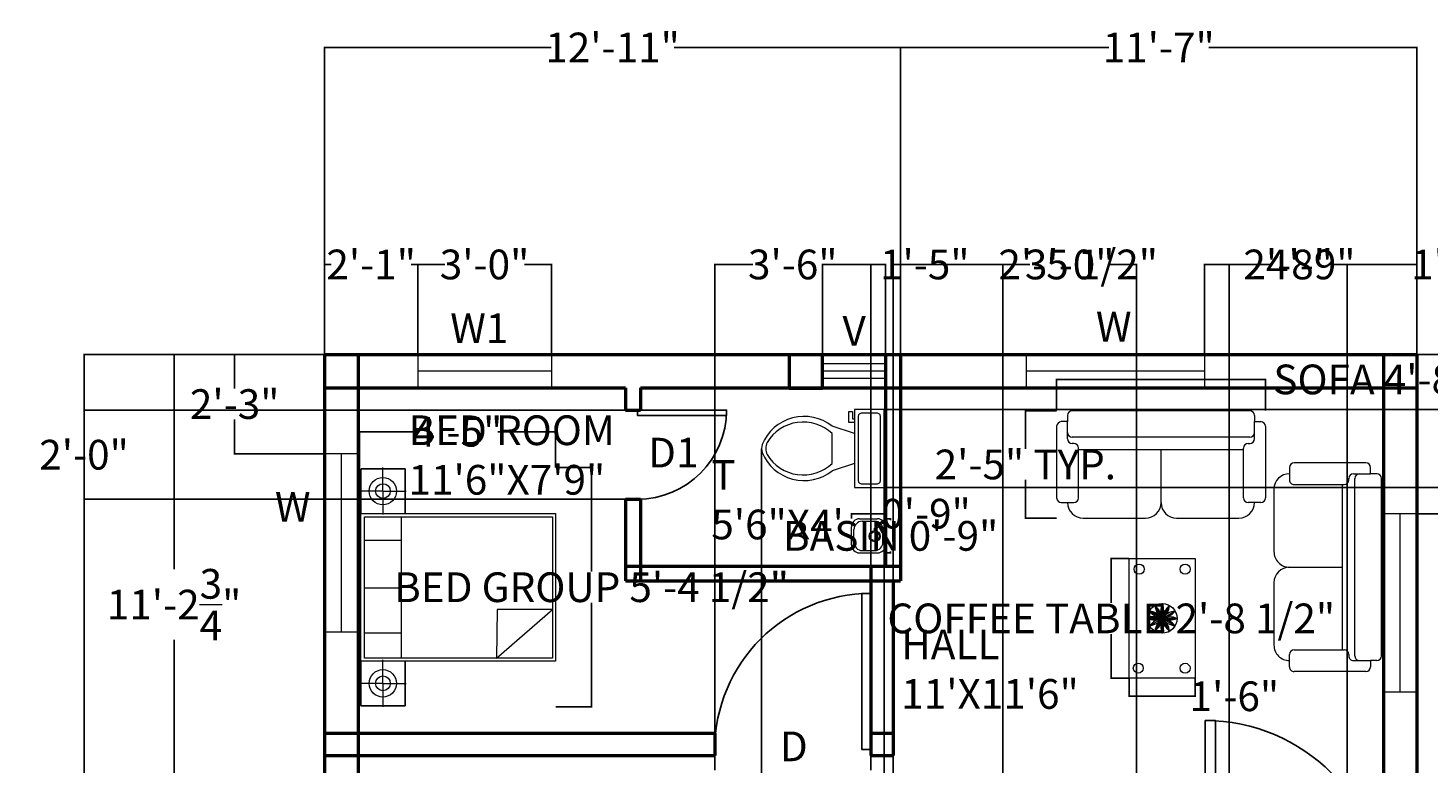
# Model space of a CAD drawing. Units: inches. Extents: x 1305 to 1889, y -508 to -5.
# Tile 7 of 8: x 1314 to 1691, y -220 to -22. Entities that reach past the tile are written whole.
import ezdxf

# ---------------------------------------------------------------- set-up
doc = ezdxf.new("R2010")
doc.units = ezdxf.units.IN
doc.header["$MEASUREMENT"] = 0
for name, color, linetype, lineweight in [('A-ANNO-DIMS', 2, 'Continuous', 18), ('A-ANNO-TEXT', 7, 'Continuous', 18), ('A-AREA-IDEN', 7, 'Continuous', 25), ('A-COLS', 7, 'Continuous', 50), ('A-DOOR', 3, 'Continuous', 25), ('A-FLOR-FIXT', 9, 'Continuous', 18), ('A-FURN', 8, 'Continuous', 18), ('A-GLAZ', 4, 'Continuous', 18), ('A-WALL', 7, 'Continuous', 50)]:
    doc.layers.add(name, color=color, linetype=linetype, lineweight=lineweight)
doc.styles.get("Standard").update_dxf_attribs({"font": 'arial.ttf', "height": 8})
doc.dimstyles.get("Standard").update_dxf_attribs({"dimtxt": 0.18, "dimasz": 0.18, "dimexe": 0.18, "dimexo": 0.0625, "dimgap": 0.09, "dimtad": 0, "dimtih": 1, "dimtoh": 1, "dimzin": 0, "dimdsep": 46, "dimlunit": 4, "dimtxsty": 'Standard', "dimcen": 0.09, "dimadec": 0, "dimazin": 0, "dimtfac": 1, "dimtofl": 0, "dimtmove": 0, "dimatfit": 3, "dimfxl": 1, "dimtolj": 1, "dimtzin": 0, "dimarcsym": 0})

# ---------------------------------------------------------------- blocks, each defined once
blk = doc.blocks.new('*U13')
for p, q in [((0, 0), (0, -100)), ((750, 0), (750, -100))]:
    blk.add_line(p, q)
blk.add_lwpolyline([(0, 0), (0, 750), (43.75, 750), (43.75, 0)], close=True)
blk.add_arc((0, 0), 750, 0, 90)
blk = doc.blocks.new('*U14')
for p, q in [((-750, 0), (-750, -100)), ((0, 0), (0, -100))]:
    blk.add_line(p, q)
blk.add_lwpolyline([(0, 0), (0, 750), (-43.75, 750), (-43.75, 0)], close=True)
blk.add_arc((0, 0), 750, 90, 180)
blk = doc.blocks.new('*U12')
for p, q in [((9.5, -6), (9.5, -2)), ((-10, -8.5), (-8, -8.5)), ((-10, -9.5), (-10, -8.5)), ((-7, -9.5), (-10, -9.5)), ((-8, -8.5), (-8, -8)), ((-7, -8), (-7, -9.5)), ((-4, -8), (-6, -14)), ((4, -8), (6, -14)), ((4, -14), (-4, -14))]:
    blk.add_line(p, q)
blk.add_lwpolyline([(10.5, -8), (10.5, 0), (-10.5, 0), (-10.5, -8)], close=True)
for points in [[(-9.5, -2), (-9.5, -6)], [(8.5, -1), (-8.5, -1)], [(-8.5, -7), (8.5, -7)]]:
    blk.add_lwpolyline(points)
for centre, radius, start, end in [((-8.62, -1.88), 0.884, 81.8699, 188.1301), ((8.62, -1.88), 0.884, 351.8699, 98.1301), ((-8.62, -6.12), 0.884, 171.8699, 278.1301), ((8.62, -6.12), 0.884, 261.8699, 8.1301), ((3.52, -21.58), 12.17, 141.4691, 247.9714), ((4.2, -21.82), 11.33, 136.3677, 238.9468), ((-3.52, -21.58), 12.17, 292.0284, 38.5307), ((-4.2, -21.82), 11.33, 301.053, 43.6321), ((0, -27.88), 4, 245.7318, 294.2682), ((0, -29), 4, 254.8605, 285.1395)]:
    blk.add_arc(centre, radius, start, end)
blk = doc.blocks.new('A$C027E3DAA')
for p, q in [((48, 356), (128, 276)), ((142, 290), (63, 369)), ((320, 420), (100, 420)), ((291, 388), (131, 388)), ((0, 100), (0, 320)), ((31, 132), (31, 288)), ((128, 276), (142, 290)), ((391, 132), (391, 288)), ((420, 100), (420, 320)), ((291, 32), (131, 32)), ((320, 0), (100, 0))]:
    blk.add_line(p, q)
for centre, radius in [((47, 373), 16.5), ((47, 373), 8.24), ((214, 287), 68.5), ((214, 287), 54.8)]:
    blk.add_circle(centre, radius)
for centre, start, end in [((100, 320), 90, 180), ((131, 288), 90, 180), ((291, 288), 0, 90), ((320, 320), 0, 90), ((100, 100), 180, 270), ((131, 132), 180, 270), ((291, 132), 270, 0), ((320, 100), 270, 0)]:
    blk.add_arc(centre, 100, start, end)
blk = doc.blocks.new('A$C214F6537')
for p, q in [((0.238, 1.755, -0.439), (0.238, 1.993, -0.439)), ((2.192, 1.755, -0.439), (2.192, 1.993, -0.439)), ((0.465, 1.98, -0.169), (0.011, 1.98, -0.169)), ((0.011, 1.98, -0.169), (0.011, 1.53, -0.169)), ((0.011, 1.98, -0.169), (2.419, 1.98, -0.169)), ((0.011, 1.53, -0.169), (0.011, 1.98, -0.169)), ((0.465, 0, -0.169), (0.465, 1.98, -0.169)), ((0.465, 1.98, -0.169), (1.965, 1.98, -0.169)), ((0.465, 1.53, -0.169), (0.465, 1.98, -0.169)), ((0.495, 1.941, -0.169), (1.929, 1.941, -0.169)), ((0.495, 1.57, -0.169), (0.495, 1.941, -0.169)), ((0.752, 1.941, -0.169), (0.752, 1.57, -0.169)), ((1.209, 1.941, -0.169), (1.209, 1.57, -0.169)), ((1.694, 1.941, -0.169), (1.694, 1.57, -0.169)), ((1.929, 1.941, -0.169), (1.929, 1.57, -0.169)), ((1.965, 1.98, -0.169), (1.965, 0, -0.169)), ((2.419, 1.98, -0.169), (1.965, 1.98, -0.169)), ((1.965, 1.98, -0.169), (1.965, 1.53, -0.169)), ((2.419, 1.53, -0.169), (2.419, 1.98, -0.169)), ((2.419, 1.98, -0.169), (2.419, 1.53, -0.169)), ((0.238, 1.755, -0.439), (0, 1.755, -0.439)), ((0.238, 1.755, -0.439), (0.238, 1.517, -0.439)), ((0.238, 1.755, -0.439), (0.476, 1.755, -0.439)), ((2.192, 1.755, -0.439), (1.954, 1.755, -0.439)), ((2.192, 1.755, -0.439), (2.43, 1.755, -0.439)), ((2.192, 1.755, -0.439), (2.192, 1.517, -0.439)), ((0.495, 0.032, -0.169), (0.495, 1.57, -0.169)), ((1.929, 1.57, -0.169), (0.495, 1.57, -0.169)), ((1.929, 1.57, -0.169), (1.929, 0.032, -0.169)), ((0.011, 1.53, -0.169), (0.465, 1.53, -0.169)), ((0.465, 1.53, -0.169), (0.011, 1.53, -0.169)), ((0.465, 0, -0.169), (0.465, 1.53, -0.169)), ((1.965, 1.53, -0.169), (2.419, 1.53, -0.169)), ((2.419, 1.53, -0.169), (1.965, 1.53, -0.169)), ((1.965, 1.53, -0.169), (1.965, 0, -0.169)), ((0.495, 0.6, -0.169), (0.987, 0.032, -0.169)), ((0.987, 0.595, -0.169), (0.495, 0.6, -0.169)), ((0.987, 0.032, -0.169), (0.987, 0.595, -0.169)), ((1.965, 0, -0.169), (0.465, 0, -0.169)), ((1.965, 0, -0.169), (0.465, 0, -0.169)), ((1.929, 0.032, -0.169), (0.495, 0.032, -0.169))]:
    blk.add_line(p, q)
for centre, radius in [((0.238, 1.755, -0.439), 0.139), ((2.192, 1.755, -0.439), 0.139), ((0.238, 1.755, -0.439), 0.075), ((2.192, 1.755, -0.439), 0.075)]:
    blk.add_circle(centre, radius)
blk = doc.blocks.new('A$C02A636C4')
for p, q in [((0.0679, 0.6401), (0.0679, 0.6013)), ((1.2026, 0.6692), (0.097, 0.6692)), ((1.2317, 0.6401), (1.2317, 0.6013)), ((0, 0.5722), (0, 0.1261)), ((0.0679, 0.6013), (0.0291, 0.6013)), ((0.0679, 0.5334), (0.0679, 0.6013)), ((0.0679, 0.4946), (0.0679, 0.5431)), ((1.2317, 0.6013), (1.2705, 0.6013)), ((1.2317, 0.5334), (1.2317, 0.6013)), ((1.2317, 0.4946), (1.2317, 0.5431)), ((1.2996, 0.5722), (1.2996, 0.1261)), ((1.2026, 0.5043), (0.097, 0.5043)), ((0.1067, 0.4655), (0.097, 0.4655)), ((0.1358, 0.1261), (0.1358, 0.4364)), ((1.1638, 0.1261), (1.1638, 0.4364)), ((1.1929, 0.4655), (1.2026, 0.4655)), ((1.1638, 0.4267), (0.1358, 0.4267)), ((0.6498, 0.097), (0.6498, 0.4267)), ((0.0291, 0.097), (0.1067, 0.097)), ((1.2705, 0.097), (1.1929, 0.097)), ((0.1649, 0), (0.5528, 0)), ((0.7468, 0), (1.1347, 0))]:
    blk.add_line(p, q)
for centre, radius, start, end in [((0.097, 0.6401), 0.0291, 90, 180), ((1.2026, 0.6401), 0.0291, 0, 90), ((0.0291, 0.5722), 0.0291, 90, 180), ((0.097, 0.5334), 0.0291, 180, 270), ((1.2026, 0.5334), 0.0291, 270, 0), ((1.2705, 0.5722), 0.0291, 0, 90), ((0.097, 0.4946), 0.0291, 180, 270), ((0.1067, 0.4364), 0.0291, 0, 90), ((1.1929, 0.4364), 0.0291, 90, 180), ((1.2026, 0.4946), 0.0291, 270, 0), ((0.0291, 0.1261), 0.0291, 180, 270), ((0.1649, 0.097), 0.097, 180, 270), ((0.1067, 0.1261), 0.0291, 270, 0), ((0.5528, 0.097), 0.097, 270, 0), ((0.7468, 0.097), 0.097, 180, 270), ((1.1347, 0.097), 0.097, 270, 0), ((1.1929, 0.1261), 0.0291, 180, 270), ((1.2705, 0.1261), 0.0291, 270, 0)]:
    blk.add_arc(centre, radius, start, end)
blk = doc.blocks.new('table')
blk.add_lwpolyline([(-20.55, 0), (36.33, 0), (36.33, -31.34), (-20.55, -31.34)], close=True)
for centre in [(-15.51, -4.83), (31.56, -4.83), (-15.51, -26.62), (31.48, -27.03)]:
    blk.add_circle(centre, 2.38)
blk = doc.blocks.new('*U18')
for p, q in [((3.98, 7.97), (3.98, 0)), ((0, 3.98), (7.97, 3.98))]:
    blk.add_line(p, q)
blk.add_circle((3.98, 3.98), 3.98)
for centre, start, end in [((8.79, 5.97), 157.5, 202.5), ((-0.82, 5.97), 337.5, 22.5), ((1.99, -0.82), 67.5, 112.5), ((1.99, 8.79), 247.5, 292.5), ((8.79, 1.99), 157.5, 202.5), ((5.97, -0.82), 67.5, 112.5), ((5.97, 8.79), 247.5, 292.5), ((-0.82, 1.99), 337.5, 22.5)]:
    blk.add_arc(centre, 5.2, start, end)
blk = doc.blocks.new('*U19')
at = {"layer": 'A-FURN', "color": 0, "linetype": 'ByBlock', "lineweight": -2, "transparency": 16777216}
for p, rotation in [((1620.98, -186.76), 60), ((1624.96, -182.78), 120), ((1618.06, -175.88), 240), ((1614.08, -179.87), 300), ((1623.5, -177.34), 180)]:
    blk.add_blockref('*U18', p, dxfattribs=dict(at, rotation=rotation))
blk.add_blockref('*U18', (1615.54, -185.31), dxfattribs=at)
blk = doc.blocks.new('*D20')
at = {"layer": 'A-ANNO-DIMS', "color": 0, "lineweight": -2, "transparency": 16777216}
for p, q in [((1394.01, -110.24), (1353.36, -110.24)), ((1353.54, -110.42), (1353.54, -168.1)), ((1353.54, -244.8), (1353.54, -187.12)), ((1394.01, -244.98), (1353.36, -244.98))]:
    blk.add_line(p, q, dxfattribs=at)
at = {"layer": 'A-ANNO-DIMS', "color": 0, "transparency": 16777216}
for points in [[(1353.51, -110.42), (1353.57, -110.42), (1353.54, -110.24)], [(1353.51, -244.8), (1353.57, -244.8), (1353.54, -244.98)]]:
    blk.add_solid(points, dxfattribs=at)
at = {"layer": 'Defpoints', "color": 0, "transparency": 16777216}
for p in [(1394.07, -110.24), (1353.54, -244.98), (1394.07, -244.98)]:
    blk.add_point(p, dxfattribs=at)
at = {"layer": 'A-ANNO-DIMS', "color": 0, "transparency": 16777216, "insert": (1353.54, -177.61), "char_height": 8, "attachment_point": 5}
blk.add_mtext('\\A1;11\'-2{\\H1x;\\S3/4;}"', dxfattribs=at)
blk = doc.blocks.new('*D25')
at = {"layer": 'A-ANNO-DIMS', "color": 0, "lineweight": -2, "transparency": 16777216}
for p, q in [((1394.07, -110.18), (1394.07, -27.4)), ((1394.25, -27.58), (1455.01, -27.58)), ((1548.89, -27.58), (1488.14, -27.58)), ((1549.07, -110.18), (1549.07, -27.4))]:
    blk.add_line(p, q, dxfattribs=at)
at = {"layer": 'A-ANNO-DIMS', "color": 0, "transparency": 16777216}
for points in [[(1394.25, -27.55), (1394.25, -27.61), (1394.07, -27.58)], [(1548.89, -27.55), (1548.89, -27.61), (1549.07, -27.58)]]:
    blk.add_solid(points, dxfattribs=at)
at = {"layer": 'Defpoints', "color": 0, "transparency": 16777216}
for p in [(1549.07, -27.58), (1394.07, -110.24), (1549.07, -110.24)]:
    blk.add_point(p, dxfattribs=at)
at = {"layer": 'A-ANNO-DIMS', "color": 0, "transparency": 16777216, "insert": (1471.57, -27.58), "char_height": 8, "attachment_point": 5}
blk.add_mtext('\\A1;12\'-11"', dxfattribs=at)
blk = doc.blocks.new('*D26')
at = {"layer": 'A-ANNO-DIMS', "color": 0, "lineweight": -2, "transparency": 16777216}
for p, q in [((1549.07, -110.18), (1549.07, -27.4)), ((1549.25, -27.58), (1605.12, -27.58)), ((1687.89, -27.58), (1632.03, -27.58)), ((1688.07, -110.18), (1688.07, -27.4))]:
    blk.add_line(p, q, dxfattribs=at)
at = {"layer": 'A-ANNO-DIMS', "color": 0, "transparency": 16777216}
for points in [[(1549.25, -27.55), (1549.25, -27.61), (1549.07, -27.58)], [(1687.89, -27.55), (1687.89, -27.61), (1688.07, -27.58)]]:
    blk.add_solid(points, dxfattribs=at)
at = {"layer": 'Defpoints', "color": 0, "transparency": 16777216}
for p in [(1688.07, -27.58), (1549.07, -110.24), (1688.07, -110.24)]:
    blk.add_point(p, dxfattribs=at)
at = {"layer": 'A-ANNO-DIMS', "color": 0, "transparency": 16777216, "insert": (1618.57, -27.58), "char_height": 8, "attachment_point": 5}
blk.add_mtext('\\A1;11\'-7"', dxfattribs=at)
blk = doc.blocks.new('WIN-48IN')
for p, q in [((0, 9), (0, 0)), ((48, 9), (48, 0)), ((48, 4.5), (0, 4.5))]:
    blk.add_line(p, q)
blk = doc.blocks.new('COL-9X9')
blk.add_lwpolyline([(0, 0), (9, 0), (9, 9), (0, 9)], close=True)
blk = doc.blocks.new('*D36')
at = {"layer": 'A-ANNO-DIMS', "color": 0, "lineweight": -2, "transparency": 16777216}
for p, q in [((1545.09, -154.5), (1546.59, -154.5)), ((1546.41, -154.68), (1546.41, -154.87)), ((1545.09, -163.69), (1546.59, -163.69)), ((1546.41, -163.51), (1546.41, -163.32))]:
    blk.add_line(p, q, dxfattribs=at)
at = {"layer": 'A-ANNO-DIMS', "color": 0, "transparency": 16777216}
for points in [[(1546.38, -154.68), (1546.44, -154.68), (1546.41, -154.5)], [(1546.38, -163.51), (1546.44, -163.51), (1546.41, -163.69)]]:
    blk.add_solid(points, dxfattribs=at)
at = {"layer": 'Defpoints', "color": 0, "transparency": 16777216}
for p in [(1545.03, -154.5), (1545.03, -163.69), (1546.41, -163.69)]:
    blk.add_point(p, dxfattribs=at)
at = {"layer": 'A-ANNO-DIMS', "color": 0, "transparency": 16777216, "insert": (1546.41, -159.1), "char_height": 8, "attachment_point": 5}
blk.add_mtext('\\A1;BASIN 0\'-9"', dxfattribs=at)
blk = doc.blocks.new('*D37')
at = {"layer": 'A-ANNO-DIMS', "color": 0, "lineweight": -2, "transparency": 16777216}
for p, q in [((1535.85, -154.44), (1535.85, -152.94)), ((1536.03, -153.12), (1544.85, -153.12)), ((1545.03, -154.44), (1545.03, -152.94)), ((1545.03, -153.12), (1545.21, -153.12))]:
    blk.add_line(p, q, dxfattribs=at)
at = {"layer": 'A-ANNO-DIMS', "color": 0, "transparency": 16777216}
for points in [[(1536.03, -153.09), (1536.03, -153.15), (1535.85, -153.12)], [(1544.85, -153.09), (1544.85, -153.15), (1545.03, -153.12)]]:
    blk.add_solid(points, dxfattribs=at)
at = {"layer": 'Defpoints', "color": 0, "transparency": 16777216}
for p in [(1545.03, -153.12), (1535.85, -154.5), (1545.03, -154.5)]:
    blk.add_point(p, dxfattribs=at)
at = {"layer": 'A-ANNO-DIMS', "color": 0, "transparency": 16777216, "insert": (1555.93, -153.12), "char_height": 8, "attachment_point": 5}
blk.add_mtext('\\A1;0\'-9"', dxfattribs=at)
blk = doc.blocks.new('*D38')
at = {"layer": 'A-ANNO-DIMS', "color": 0, "lineweight": -2, "transparency": 16777216}
for p, q in [((1591.1, -125.34), (1591.1, -116.79)), ((1647.29, -125.34), (1647.29, -116.79)), ((1591.28, -116.97), (1647.11, -116.97)), ((1647.29, -116.97), (1647.47, -116.97))]:
    blk.add_line(p, q, dxfattribs=at)
at = {"layer": 'A-ANNO-DIMS', "color": 0, "transparency": 16777216}
for points in [[(1591.28, -116.94), (1591.28, -117), (1591.1, -116.97)], [(1647.11, -116.94), (1647.11, -117), (1647.29, -116.97)]]:
    blk.add_solid(points, dxfattribs=at)
at = {"layer": 'Defpoints', "color": 0, "transparency": 16777216}
for p in [(1647.29, -116.97), (1591.1, -125.4), (1647.29, -125.4)]:
    blk.add_point(p, dxfattribs=at)
at = {"layer": 'A-ANNO-DIMS', "color": 0, "transparency": 16777216, "insert": (1688.69, -116.97), "char_height": 8, "attachment_point": 5}
blk.add_mtext('\\A1;SOFA 4\'-8" TYP.', dxfattribs=at)
blk = doc.blocks.new('*D39')
at = {"layer": 'A-ANNO-DIMS', "color": 0, "lineweight": -2, "transparency": 16777216}
for p, q in [((1591.04, -125.4), (1582.49, -125.4)), ((1582.67, -125.58), (1582.67, -135.7)), ((1582.67, -154.16), (1582.67, -144.04)), ((1591.04, -154.34), (1582.49, -154.34))]:
    blk.add_line(p, q, dxfattribs=at)
at = {"layer": 'A-ANNO-DIMS', "color": 0, "transparency": 16777216}
for points in [[(1582.64, -125.58), (1582.7, -125.58), (1582.67, -125.4)], [(1582.64, -154.16), (1582.7, -154.16), (1582.67, -154.34)]]:
    blk.add_solid(points, dxfattribs=at)
at = {"layer": 'Defpoints', "color": 0, "transparency": 16777216}
for p in [(1582.67, -125.4), (1591.1, -125.4), (1591.1, -154.34)]:
    blk.add_point(p, dxfattribs=at)
at = {"layer": 'A-ANNO-DIMS', "color": 0, "transparency": 16777216, "insert": (1582.67, -139.87), "char_height": 8, "attachment_point": 5}
blk.add_mtext('\\A1;2\'-5" TYP.', dxfattribs=at)
blk = doc.blocks.new('*D46')
at = {"layer": 'A-ANNO-DIMS', "color": 0, "lineweight": -2, "transparency": 16777216}
for p, q in [((1456.31, -140.72), (1466.09, -140.72)), ((1465.91, -140.9), (1465.91, -168.69)), ((1465.91, -204.93), (1465.91, -177.15)), ((1456.31, -205.11), (1466.09, -205.11))]:
    blk.add_line(p, q, dxfattribs=at)
at = {"layer": 'A-ANNO-DIMS', "color": 0, "transparency": 16777216}
for points in [[(1465.88, -140.9), (1465.94, -140.9), (1465.91, -140.72)], [(1465.88, -204.93), (1465.94, -204.93), (1465.91, -205.11)]]:
    blk.add_solid(points, dxfattribs=at)
at = {"layer": 'Defpoints', "color": 0, "transparency": 16777216}
for p in [(1456.25, -140.72), (1465.91, -140.72), (1456.25, -205.11)]:
    blk.add_point(p, dxfattribs=at)
at = {"layer": 'A-ANNO-DIMS', "color": 0, "transparency": 16777216, "insert": (1465.91, -172.92), "char_height": 8, "attachment_point": 5}
blk.add_mtext('\\A1;BED GROUP 5\'-4 1/2"', dxfattribs=at)
blk = doc.blocks.new('*D47')
at = {"layer": 'A-ANNO-DIMS', "color": 0, "lineweight": -2, "transparency": 16777216}
for p, q in [((1403.43, -140.66), (1403.43, -130.88)), ((1403.61, -131.06), (1418.96, -131.06)), ((1456.07, -131.06), (1440.73, -131.06)), ((1456.25, -140.66), (1456.25, -130.88))]:
    blk.add_line(p, q, dxfattribs=at)
at = {"layer": 'A-ANNO-DIMS', "color": 0, "transparency": 16777216}
for points in [[(1403.61, -131.03), (1403.61, -131.09), (1403.43, -131.06)], [(1456.07, -131.03), (1456.07, -131.09), (1456.25, -131.06)]]:
    blk.add_solid(points, dxfattribs=at)
at = {"layer": 'Defpoints', "color": 0, "transparency": 16777216}
for p in [(1403.43, -131.06), (1403.43, -140.72), (1456.25, -140.72)]:
    blk.add_point(p, dxfattribs=at)
at = {"layer": 'A-ANNO-DIMS', "color": 0, "transparency": 16777216, "insert": (1429.84, -131.06), "char_height": 8, "attachment_point": 5}
blk.add_mtext('\\A1;4\'-5"', dxfattribs=at)
blk = doc.blocks.new('*D48')
at = {"layer": 'A-ANNO-DIMS', "color": 0, "lineweight": -2, "transparency": 16777216}
for p, q in [((1610.57, -165.2), (1605.61, -165.2)), ((1605.79, -165.38), (1605.79, -177.09)), ((1605.79, -197.27), (1605.79, -185.55)), ((1610.57, -197.45), (1605.61, -197.45))]:
    blk.add_line(p, q, dxfattribs=at)
at = {"layer": 'A-ANNO-DIMS', "color": 0, "transparency": 16777216}
for points in [[(1605.76, -165.38), (1605.82, -165.38), (1605.79, -165.2)], [(1605.76, -197.27), (1605.82, -197.27), (1605.79, -197.45)]]:
    blk.add_solid(points, dxfattribs=at)
at = {"layer": 'Defpoints', "color": 0, "transparency": 16777216}
for p in [(1610.63, -165.2), (1605.79, -197.45), (1610.63, -197.45)]:
    blk.add_point(p, dxfattribs=at)
at = {"layer": 'A-ANNO-DIMS', "color": 0, "transparency": 16777216, "insert": (1605.79, -181.32), "char_height": 8, "attachment_point": 5}
blk.add_mtext('\\A1;COFFEE TABLE 2\'-8 1/2"', dxfattribs=at)
blk = doc.blocks.new('*D49')
at = {"layer": 'A-ANNO-DIMS', "color": 0, "lineweight": -2, "transparency": 16777216}
for p, q in [((1610.63, -197.51), (1610.63, -202.47)), ((1628.41, -197.51), (1628.41, -202.47)), ((1610.81, -202.29), (1628.23, -202.29)), ((1628.41, -202.29), (1628.59, -202.29))]:
    blk.add_line(p, q, dxfattribs=at)
at = {"layer": 'A-ANNO-DIMS', "color": 0, "transparency": 16777216}
for points in [[(1610.81, -202.26), (1610.81, -202.32), (1610.63, -202.29)], [(1628.23, -202.26), (1628.23, -202.32), (1628.41, -202.29)]]:
    blk.add_solid(points, dxfattribs=at)
at = {"layer": 'Defpoints', "color": 0, "transparency": 16777216}
for p in [(1610.63, -197.45), (1628.41, -197.45), (1628.41, -202.29)]:
    blk.add_point(p, dxfattribs=at)
at = {"layer": 'A-ANNO-DIMS', "color": 0, "transparency": 16777216, "insert": (1638.93, -202.29), "char_height": 8, "attachment_point": 5}
blk.add_mtext('\\A1;1\'-6"', dxfattribs=at)
blk = doc.blocks.new('*D51')
at = {"layer": 'A-ANNO-DIMS', "color": 0, "lineweight": -2, "transparency": 16777216}
for p, q in [((1394.01, -110.24), (1329.13, -110.24)), ((1329.31, -110.42), (1329.31, -281.56)), ((1329.31, -461.06), (1329.31, -289.92)), ((1394.01, -461.24), (1329.13, -461.24))]:
    blk.add_line(p, q, dxfattribs=at)
at = {"layer": 'A-ANNO-DIMS', "color": 0, "transparency": 16777216}
for points in [[(1329.28, -110.42), (1329.34, -110.42), (1329.31, -110.24)], [(1329.28, -461.06), (1329.34, -461.06), (1329.31, -461.24)]]:
    blk.add_solid(points, dxfattribs=at)
at = {"layer": 'Defpoints', "color": 0, "transparency": 16777216}
for p in [(1394.07, -110.24), (1329.31, -461.24), (1394.07, -461.24)]:
    blk.add_point(p, dxfattribs=at)
at = {"layer": 'A-ANNO-DIMS', "color": 0, "transparency": 16777216, "insert": (1329.31, -285.74), "char_height": 8, "attachment_point": 5}
blk.add_mtext('\\A1;29\'-3"', dxfattribs=at)
blk = doc.blocks.new('*D52')
at = {"layer": 'A-ANNO-DIMS', "color": 0, "lineweight": -2, "transparency": 16777216}
for p, q in [((1479.01, -125.24), (1329.13, -125.24)), ((1329.31, -125.42), (1329.31, -133.06)), ((1329.31, -149.06), (1329.31, -141.41)), ((1479.01, -149.24), (1329.13, -149.24))]:
    blk.add_line(p, q, dxfattribs=at)
at = {"layer": 'A-ANNO-DIMS', "color": 0, "transparency": 16777216}
for points in [[(1329.28, -125.42), (1329.34, -125.42), (1329.31, -125.24)], [(1329.28, -149.06), (1329.34, -149.06), (1329.31, -149.24)]]:
    blk.add_solid(points, dxfattribs=at)
at = {"layer": 'Defpoints', "color": 0, "transparency": 16777216}
for p in [(1479.07, -125.24), (1329.31, -149.24), (1479.07, -149.24)]:
    blk.add_point(p, dxfattribs=at)
at = {"layer": 'A-ANNO-DIMS', "color": 0, "transparency": 16777216, "insert": (1329.31, -137.24), "char_height": 8, "attachment_point": 5}
blk.add_mtext('\\A1;2\'-0"', dxfattribs=at)
blk = doc.blocks.new('*D53')
at = {"layer": 'A-ANNO-DIMS', "color": 0, "lineweight": -2, "transparency": 16777216}
for p, q in [((1528.11, -110.24), (1528.11, -85.83)), ((1528.29, -86.01), (1544.89, -86.01)), ((1545.07, -110.18), (1545.07, -85.83)), ((1545.07, -86.01), (1545.25, -86.01))]:
    blk.add_line(p, q, dxfattribs=at)
at = {"layer": 'A-ANNO-DIMS', "color": 0, "transparency": 16777216}
for points in [[(1528.29, -85.98), (1528.29, -86.04), (1528.11, -86.01)], [(1544.89, -85.98), (1544.89, -86.04), (1545.07, -86.01)]]:
    blk.add_solid(points, dxfattribs=at)
at = {"layer": 'Defpoints', "color": 0, "transparency": 16777216}
for p in [(1545.07, -86.01), (1528.11, -110.3), (1545.07, -110.24)]:
    blk.add_point(p, dxfattribs=at)
at = {"layer": 'A-ANNO-DIMS', "color": 0, "transparency": 16777216, "insert": (1555.6, -86.01), "char_height": 8, "attachment_point": 5}
blk.add_mtext('\\A1;1\'-5"', dxfattribs=at)
blk = doc.blocks.new('*D54')
at = {"layer": 'A-ANNO-DIMS', "color": 0, "lineweight": -2, "transparency": 16777216}
for p, q in [((1544.74, -125.07), (1712.53, -125.07)), ((1712.35, -125.25), (1712.35, -131.39)), ((1712.35, -145.89), (1712.35, -139.74)), ((1544.74, -146.07), (1712.53, -146.07))]:
    blk.add_line(p, q, dxfattribs=at)
at = {"layer": 'A-ANNO-DIMS', "color": 0, "transparency": 16777216}
for points in [[(1712.32, -125.25), (1712.38, -125.25), (1712.35, -125.07)], [(1712.32, -145.89), (1712.38, -145.89), (1712.35, -146.07)]]:
    blk.add_solid(points, dxfattribs=at)
at = {"layer": 'Defpoints', "color": 0, "transparency": 16777216}
for p in [(1544.68, -125.07), (1544.68, -146.07), (1712.35, -146.07)]:
    blk.add_point(p, dxfattribs=at)
at = {"layer": 'A-ANNO-DIMS', "color": 0, "transparency": 16777216, "insert": (1712.35, -135.57), "char_height": 8, "attachment_point": 5}
blk.add_mtext('\\A1;1\'-9"', dxfattribs=at)
blk = doc.blocks.new('*D55')
at = {"layer": 'A-ANNO-DIMS', "color": 0, "lineweight": -2, "transparency": 16777216}
for p, q in [((1511.68, -135.63), (1511.68, -493.26)), ((1544.68, -146.13), (1544.68, -493.26)), ((1511.86, -493.08), (1517.39, -493.08)), ((1544.5, -493.08), (1538.97, -493.08))]:
    blk.add_line(p, q, dxfattribs=at)
at = {"layer": 'A-ANNO-DIMS', "color": 0, "transparency": 16777216}
for points in [[(1511.86, -493.05), (1511.86, -493.11), (1511.68, -493.08)], [(1544.5, -493.05), (1544.5, -493.11), (1544.68, -493.08)]]:
    blk.add_solid(points, dxfattribs=at)
at = {"layer": 'Defpoints', "color": 0, "transparency": 16777216}
for p in [(1511.68, -135.57), (1544.68, -146.07), (1544.68, -493.08)]:
    blk.add_point(p, dxfattribs=at)
at = {"layer": 'A-ANNO-DIMS', "color": 0, "transparency": 16777216, "insert": (1528.18, -493.08), "char_height": 8, "attachment_point": 5}
blk.add_mtext('\\A1;2\'-9"', dxfattribs=at)
blk = doc.blocks.new('*D56')
at = {"layer": 'A-ANNO-DIMS', "color": 0, "lineweight": -2, "transparency": 16777216}
for p, q in [((1419.11, -110.18), (1419.11, -85.83)), ((1419.29, -86.01), (1426.39, -86.01)), ((1454.93, -86.01), (1447.83, -86.01)), ((1455.11, -110.18), (1455.11, -85.83))]:
    blk.add_line(p, q, dxfattribs=at)
at = {"layer": 'A-ANNO-DIMS', "color": 0, "transparency": 16777216}
for points in [[(1419.29, -85.98), (1419.29, -86.04), (1419.11, -86.01)], [(1454.93, -85.98), (1454.93, -86.04), (1455.11, -86.01)]]:
    blk.add_solid(points, dxfattribs=at)
at = {"layer": 'Defpoints', "color": 0, "transparency": 16777216}
for p in [(1455.11, -86.01), (1419.11, -110.24), (1455.11, -110.24)]:
    blk.add_point(p, dxfattribs=at)
at = {"layer": 'A-ANNO-DIMS', "color": 0, "transparency": 16777216, "insert": (1437.11, -86.01), "char_height": 8, "attachment_point": 5}
blk.add_mtext('\\A1;3\'-0"', dxfattribs=at)
blk = doc.blocks.new('*D57')
at = {"layer": 'A-ANNO-DIMS', "color": 0, "lineweight": -2, "transparency": 16777216}
for p, q in [((1394.07, -110.18), (1394.07, -85.83)), ((1394.25, -86.01), (1395.8, -86.01)), ((1418.93, -86.01), (1417.38, -86.01)), ((1419.11, -110.18), (1419.11, -85.83))]:
    blk.add_line(p, q, dxfattribs=at)
at = {"layer": 'A-ANNO-DIMS', "color": 0, "transparency": 16777216}
for points in [[(1394.25, -85.98), (1394.25, -86.04), (1394.07, -86.01)], [(1418.93, -85.98), (1418.93, -86.04), (1419.11, -86.01)]]:
    blk.add_solid(points, dxfattribs=at)
at = {"layer": 'Defpoints', "color": 0, "transparency": 16777216}
for p in [(1419.11, -86.01), (1394.07, -110.24), (1419.11, -110.24)]:
    blk.add_point(p, dxfattribs=at)
at = {"layer": 'A-ANNO-DIMS', "color": 0, "transparency": 16777216, "insert": (1406.59, -86.01), "char_height": 8, "attachment_point": 5}
blk.add_mtext('\\A1;2\'-1"', dxfattribs=at)
blk = doc.blocks.new('*D58')
at = {"layer": 'A-ANNO-DIMS', "color": 0, "lineweight": -2, "transparency": 16777216}
for p, q in [((1630.91, -110.18), (1630.91, -85.83)), ((1631.09, -86.01), (1648.61, -86.01)), ((1687.89, -86.01), (1670.38, -86.01)), ((1688.07, -110.18), (1688.07, -85.83))]:
    blk.add_line(p, q, dxfattribs=at)
at = {"layer": 'A-ANNO-DIMS', "color": 0, "transparency": 16777216}
for points in [[(1631.09, -85.98), (1631.09, -86.04), (1630.91, -86.01)], [(1687.89, -85.98), (1687.89, -86.04), (1688.07, -86.01)]]:
    blk.add_solid(points, dxfattribs=at)
at = {"layer": 'Defpoints', "color": 0, "transparency": 16777216}
for p in [(1688.07, -86.01), (1630.91, -110.24), (1688.07, -110.24)]:
    blk.add_point(p, dxfattribs=at)
at = {"layer": 'A-ANNO-DIMS', "color": 0, "transparency": 16777216, "insert": (1659.49, -86.01), "char_height": 8, "attachment_point": 5}
blk.add_mtext('\\A1;4\'-9"', dxfattribs=at)
blk = doc.blocks.new('*D59')
at = {"layer": 'A-ANNO-DIMS', "color": 0, "lineweight": -2, "transparency": 16777216}
for p, q in [((1499.07, -212.18), (1499.07, -85.83)), ((1499.25, -86.01), (1509.35, -86.01)), ((1540.89, -86.01), (1530.79, -86.01)), ((1541.07, -212.18), (1541.07, -85.83))]:
    blk.add_line(p, q, dxfattribs=at)
at = {"layer": 'A-ANNO-DIMS', "color": 0, "transparency": 16777216}
for points in [[(1499.25, -85.98), (1499.25, -86.04), (1499.07, -86.01)], [(1540.89, -85.98), (1540.89, -86.04), (1541.07, -86.01)]]:
    blk.add_solid(points, dxfattribs=at)
at = {"layer": 'Defpoints', "color": 0, "transparency": 16777216}
for p in [(1541.07, -86.01), (1499.07, -212.24), (1541.07, -212.24)]:
    blk.add_point(p, dxfattribs=at)
at = {"layer": 'A-ANNO-DIMS', "color": 0, "transparency": 16777216, "insert": (1520.07, -86.01), "char_height": 8, "attachment_point": 5}
blk.add_mtext('\\A1;3\'-6"', dxfattribs=at)
blk = doc.blocks.new('*D63')
at = {"layer": 'A-ANNO-DIMS', "color": 0, "lineweight": -2, "transparency": 16777216}
for p, q in [((1637.53, -461.18), (1637.53, -85.83)), ((1637.71, -86.01), (1642.61, -86.01)), ((1669.11, -86.01), (1664.2, -86.01)), ((1669.29, -461.18), (1669.29, -85.83))]:
    blk.add_line(p, q, dxfattribs=at)
at = {"layer": 'A-ANNO-DIMS', "color": 0, "transparency": 16777216}
for points in [[(1637.71, -85.98), (1637.71, -86.04), (1637.53, -86.01)], [(1669.11, -85.98), (1669.11, -86.04), (1669.29, -86.01)]]:
    blk.add_solid(points, dxfattribs=at)
at = {"layer": 'Defpoints', "color": 0, "transparency": 16777216}
for p in [(1669.29, -86.01), (1637.53, -461.24), (1669.29, -461.24)]:
    blk.add_point(p, dxfattribs=at)
at = {"layer": 'A-ANNO-DIMS', "color": 0, "transparency": 16777216, "insert": (1653.41, -86.01), "char_height": 8, "attachment_point": 5}
blk.add_mtext('\\A1;2\'-8"', dxfattribs=at)
blk = doc.blocks.new('*D64')
at = {"layer": 'A-ANNO-DIMS', "color": 0, "lineweight": -2, "transparency": 16777216}
for p, q in [((1669.29, -461.18), (1669.29, -85.83)), ((1669.47, -86.01), (1687.87, -86.01)), ((1688.05, -461.23), (1688.05, -85.83)), ((1688.05, -86.01), (1688.23, -86.01))]:
    blk.add_line(p, q, dxfattribs=at)
at = {"layer": 'A-ANNO-DIMS', "color": 0, "transparency": 16777216}
for points in [[(1669.47, -85.98), (1669.47, -86.04), (1669.29, -86.01)], [(1687.87, -85.98), (1687.87, -86.04), (1688.05, -86.01)]]:
    blk.add_solid(points, dxfattribs=at)
at = {"layer": 'Defpoints', "color": 0, "transparency": 16777216}
for p in [(1688.05, -86.01), (1669.29, -461.24), (1688.05, -461.3)]:
    blk.add_point(p, dxfattribs=at)
at = {"layer": 'A-ANNO-DIMS', "color": 0, "transparency": 16777216, "insert": (1698.58, -86.01), "char_height": 8, "attachment_point": 5}
blk.add_mtext('\\A1;1\'-7"', dxfattribs=at)
blk = doc.blocks.new('*D65')
at = {"layer": 'A-ANNO-DIMS', "color": 0, "lineweight": -2, "transparency": 16777216}
for p, q in [((1394.01, -110.24), (1369.67, -110.24)), ((1369.85, -110.42), (1369.85, -119.44)), ((1369.85, -136.81), (1369.85, -127.79)), ((1394.01, -136.99), (1369.67, -136.99))]:
    blk.add_line(p, q, dxfattribs=at)
at = {"layer": 'A-ANNO-DIMS', "color": 0, "transparency": 16777216}
for points in [[(1369.82, -110.42), (1369.88, -110.42), (1369.85, -110.24)], [(1369.82, -136.81), (1369.88, -136.81), (1369.85, -136.99)]]:
    blk.add_solid(points, dxfattribs=at)
at = {"layer": 'Defpoints', "color": 0, "transparency": 16777216}
for p in [(1369.85, -110.24), (1394.07, -110.24), (1394.07, -136.99)]:
    blk.add_point(p, dxfattribs=at)
at = {"layer": 'A-ANNO-DIMS', "color": 0, "transparency": 16777216, "insert": (1369.85, -123.61), "char_height": 8, "attachment_point": 5}
blk.add_mtext('\\A1;2\'-3"', dxfattribs=at)
blk = doc.blocks.new('*D67')
at = {"layer": 'A-ANNO-DIMS', "color": 0, "lineweight": -2, "transparency": 16777216}
for p, q in [((1688.14, -110.24), (1712.53, -110.24)), ((1712.35, -110.42), (1712.35, -127.51)), ((1712.35, -152.96), (1712.35, -135.87)), ((1688.14, -153.14), (1712.53, -153.14))]:
    blk.add_line(p, q, dxfattribs=at)
at = {"layer": 'A-ANNO-DIMS', "color": 0, "transparency": 16777216}
for points in [[(1712.32, -110.42), (1712.38, -110.42), (1712.35, -110.24)], [(1712.32, -152.96), (1712.38, -152.96), (1712.35, -153.14)]]:
    blk.add_solid(points, dxfattribs=at)
at = {"layer": 'Defpoints', "color": 0, "transparency": 16777216}
for p in [(1688.07, -110.24), (1688.07, -153.14), (1712.35, -153.14)]:
    blk.add_point(p, dxfattribs=at)
at = {"layer": 'A-ANNO-DIMS', "color": 0, "transparency": 16777216, "insert": (1712.35, -131.69), "char_height": 8, "attachment_point": 5}
blk.add_mtext('\\A1;3\'-7"', dxfattribs=at)
blk = doc.blocks.new('*D69')
at = {"layer": 'A-ANNO-DIMS', "color": 0, "lineweight": -2, "transparency": 16777216}
for p, q in [((1547.07, -377.18), (1547.07, -85.83)), ((1547.25, -86.01), (1576.42, -86.01)), ((1576.6, -377.18), (1576.6, -85.83)), ((1576.6, -86.01), (1576.78, -86.01))]:
    blk.add_line(p, q, dxfattribs=at)
at = {"layer": 'A-ANNO-DIMS', "color": 0, "transparency": 16777216}
for points in [[(1547.25, -85.98), (1547.25, -86.04), (1547.07, -86.01)], [(1576.42, -85.98), (1576.42, -86.04), (1576.6, -86.01)]]:
    blk.add_solid(points, dxfattribs=at)
at = {"layer": 'Defpoints', "color": 0, "transparency": 16777216}
for p in [(1576.6, -86.01), (1547.07, -377.24), (1576.6, -377.24)]:
    blk.add_point(p, dxfattribs=at)
at = {"layer": 'A-ANNO-DIMS', "color": 0, "transparency": 16777216, "insert": (1596.89, -86.01), "char_height": 8, "attachment_point": 5}
blk.add_mtext('\\A1;2\'-5 1/2"', dxfattribs=at)
blk = doc.blocks.new('*D70')
at = {"layer": 'A-ANNO-DIMS', "color": 0, "lineweight": -2, "transparency": 16777216}
for p, q in [((1576.6, -377.18), (1576.6, -85.83)), ((1576.78, -86.01), (1583.88, -86.01)), ((1612.42, -86.01), (1605.32, -86.01)), ((1612.6, -377.18), (1612.6, -85.83))]:
    blk.add_line(p, q, dxfattribs=at)
at = {"layer": 'A-ANNO-DIMS', "color": 0, "transparency": 16777216}
for points in [[(1576.78, -85.98), (1576.78, -86.04), (1576.6, -86.01)], [(1612.42, -85.98), (1612.42, -86.04), (1612.6, -86.01)]]:
    blk.add_solid(points, dxfattribs=at)
at = {"layer": 'Defpoints', "color": 0, "transparency": 16777216}
for p in [(1612.6, -86.01), (1576.6, -377.24), (1612.6, -377.24)]:
    blk.add_point(p, dxfattribs=at)
at = {"layer": 'A-ANNO-DIMS', "color": 0, "transparency": 16777216, "insert": (1594.6, -86.01), "char_height": 8, "attachment_point": 5}
blk.add_mtext('\\A1;3\'-0"', dxfattribs=at)

msp = doc.modelspace()

# ---------------------------------------------------------------- linework, layer by layer
at = {"layer": 'A-GLAZ'}
for p, q in [((1419.11, -110.239), (1419.11, -119.239)), ((1455.11, -110.239), (1455.11, -119.239)), ((1528.11, -112.668), (1545.074, -112.668)), ((1455.11, -114.739), (1419.11, -114.739)), ((1528.11, -114.668), (1545.074, -114.668)), ((1528.11, -116.668), (1545.074, -116.668))]:
    msp.add_line(p, q, dxfattribs=at)
at = {"layer": 'A-WALL'}
for p, q in [((1394.074, -110.239), (1394.074, -461.239)), ((1394.074, -110.239), (1688.074, -110.239)), ((1403.074, -110.239), (1403.074, -389.239)), ((1545.074, -110.239), (1545.074, -167.239)), ((1549.074, -110.239), (1549.074, -171.239)), ((1679.074, -110.239), (1679.074, -461.239)), ((1688.074, -110.239), (1688.074, -461.239)), ((1394.074, -119.239), (1475.074, -119.239)), ((1475.074, -119.239), (1475.074, -125.239)), ((1479.074, -119.239), (1479.074, -125.239)), ((1479.074, -119.239), (1688.074, -119.239)), ((1475.074, -125.239), (1479.074, -125.239)), ((1475.074, -149.239), (1479.074, -149.239)), ((1475.074, -149.239), (1475.074, -171.239)), ((1479.074, -149.239), (1479.074, -171.239)), ((1475.074, -167.239), (1549.074, -167.239)), ((1541.074, -167.239), (1541.074, -218.239)), ((1475.074, -171.239), (1549.074, -171.239)), ((1547.074, -171.239), (1547.074, -218.239)), ((1394.074, -212.239), (1499.074, -212.239)), ((1499.074, -212.239), (1499.074, -218.239)), ((1541.074, -212.239), (1547.074, -212.239)), ((1394.074, -218.239), (1499.074, -218.239)), ((1541.074, -218.239), (1547.074, -218.239))]:
    msp.add_line(p, q, dxfattribs=at)

# ---------------------------------------------------------------- block references
at = {"layer": 'A-COLS'}
msp.add_blockref('COL-9X9', (1519.11, -119.301), dxfattribs=at)
at = {"layer": 'A-DOOR', "xscale": 0.0319999999999999, "yscale": 0.0319999999999999, "zscale": 0.0319999999999999, "rotation": 270}
msp.add_blockref('*U13', (1478.274, -125.239), dxfattribs=at)
at = {"layer": 'A-DOOR'}
for name, p, xscale, yscale, zscale in [('*U14', (1541.074, -216.594), 0.056, 0.056, 0.056), ('*U13', (1631.074, -256.839), 0.0640000000000004, 0.0640000000000004, 0.0640000000000004)]:
    msp.add_blockref(name, p, dxfattribs=dict(at, xscale=xscale, yscale=yscale, zscale=zscale))
at = {"layer": 'A-FLOR-FIXT', "rotation": 270}
msp.add_blockref('*U12', (1544.679, -135.569), dxfattribs=at)
at = {"layer": 'A-FLOR-FIXT', "xscale": 0.0218707690273435, "yscale": 0.0218707690273435, "zscale": 0.0218707690273435, "rotation": 270}
msp.add_blockref('A$C027E3DAA', (1535.851, -154.502), dxfattribs=at)
at = {"layer": 'A-FURN', "xscale": 43.23597249474661, "yscale": 43.23597249474661, "zscale": 43.23597249474661}
msp.add_blockref('A$C02A636C4', (1591.1, -154.337), dxfattribs=at)
at = {"layer": 'A-FURN'}
for name, p, xscale, yscale, zscale, rotation in [('A$C214F6537', (1456.252, -205.113, 4.471), 26.49727388936412, 26.49727388936412, 26.49727388936412, 89.99999999999999), ('A$C02A636C4', (1649.586, -139.434), 43.23597249474661, 43.23597249474661, 43.23597249474661, 270), ('table', (1628.407, -176.851), 0.5671065675264959, 0.5671065675264959, 0.5671065675264959, 270)]:
    msp.add_blockref(name, p, dxfattribs=dict(at, xscale=xscale, yscale=yscale, zscale=zscale, rotation=rotation))
msp.add_blockref('*U19', (0, 0), dxfattribs=at)
at = {"layer": 'A-GLAZ'}
msp.add_blockref('WIN-48IN', (1582.912, -119.239), dxfattribs=at)
at = {"layer": 'A-GLAZ', "rotation": 269.9999999999999}
for p in [(1394.074, -136.991), (1679.074, -153.141)]:
    msp.add_blockref('WIN-48IN', p, dxfattribs=at)

# ---------------------------------------------------------------- texts
at = {"layer": 'A-ANNO-TEXT', "char_height": 8, "attachment_point": 1}
for s, insert in [('W1', (1427.875, -99.201)), ('V', (1533.447, -99.891)), ('W', (1601.679, -98.764)), ('D1', (1481.128, -132.679)), ('W', (1380.699, -147.315)), ('D', (1516.592, -211.788))]:
    msp.add_mtext_dynamic_manual_height_columns(s, width=13.3749, gutter_width=40, heights=[0], dxfattribs=dict(at, insert=insert))
at = {"layer": 'A-AREA-IDEN', "char_height": 8, "attachment_point": 1}
for s, insert in [('BED ROOM\\P11\'6"X7\'9"', (1416.639, -126.661)), ('T\\P5\'6"X4\'', (1498.147, -138.695)), ('HALL\\P11\'X11\'6"', (1549.274, -184.327))]:
    msp.add_mtext_dynamic_manual_height_columns(s, width=69.27903, gutter_width=40, heights=[0], dxfattribs=dict(at, insert=insert))

# ---------------------------------------------------------------- dimensions: what is measured, and where the dimension line sits
at = {"layer": 'A-ANNO-DIMS'}
for base, p1, p2, override, picture, middle in [((1549.074, -27.58), (1394.074, -110.239), (1549.074, -110.239), {"dimclrd": 0, "dimclre": 0, "dimclrt": 0}, '*D25', (1471.574, -27.58)), ((1688.074, -27.58), (1549.074, -110.239), (1688.074, -110.239), {"dimclrd": 0, "dimclre": 0, "dimclrt": 0}, '*D26', (1618.574, -27.58)), ((1576.598, -86.014), (1547.074, -377.239), (1576.598, -377.239), {"dimdec": 1, "dimlfac": 1, "dimrnd": 0, "dimzin": 1, "dimdsep": 46, "dimlunit": 4, "dimfrac": 2}, '*D69', (1596.889, -86.014)), ((1419.11, -86.014), (1394.074, -110.239), (1419.11, -110.239), {"dimdec": 1, "dimlfac": 1, "dimrnd": 0, "dimzin": 1, "dimdsep": 46, "dimlunit": 4, "dimfrac": 2}, '*D57', (1406.592, -86.014)), ((1455.11, -86.014), (1419.11, -110.239), (1455.11, -110.239), {"dimdec": 1, "dimlfac": 1, "dimrnd": 0, "dimzin": 1, "dimdsep": 46, "dimlunit": 4, "dimfrac": 2}, '*D56', (1437.11, -86.014)), ((1541.074, -86.014), (1499.074, -212.239), (1541.074, -212.239), {"dimdec": 1, "dimlfac": 1, "dimrnd": 0, "dimzin": 1, "dimdsep": 46, "dimlunit": 4, "dimfrac": 2}, '*D59', (1520.074, -86.014)), ((1545.074, -86.014), (1528.11, -110.301), (1545.074, -110.239), {"dimdec": 1, "dimlfac": 1, "dimrnd": 0, "dimzin": 1, "dimdsep": 46, "dimlunit": 4, "dimfrac": 2}, '*D53', (1555.601, -86.014)), ((1612.598, -86.014), (1576.598, -377.239), (1612.598, -377.239), {"dimdec": 1, "dimlfac": 1, "dimrnd": 0, "dimzin": 1, "dimdsep": 46, "dimlunit": 4, "dimfrac": 2}, '*D70', (1594.598, -86.014)), ((1688.074, -86.014), (1630.912, -110.239), (1688.074, -110.239), {"dimdec": 1, "dimlfac": 1, "dimrnd": 0, "dimzin": 1, "dimdsep": 46, "dimlunit": 4, "dimfrac": 2}, '*D58', (1659.493, -86.014)), ((1669.285, -86.014), (1637.526, -461.239), (1669.285, -461.239), {"dimdec": 1, "dimlfac": 1, "dimrnd": 0, "dimzin": 1, "dimdsep": 46, "dimlunit": 4, "dimfrac": 2}, '*D63', (1653.406, -86.014)), ((1688.053, -86.014), (1669.285, -461.239), (1688.053, -461.295), {"dimdec": 1, "dimlfac": 1, "dimrnd": 0, "dimzin": 1, "dimdsep": 46, "dimlunit": 4, "dimfrac": 2}, '*D64', (1698.58, -86.014)), ((1544.679, -493.076), (1511.679, -135.569), (1544.679, -146.069), {"dimdec": 1, "dimlfac": 1, "dimrnd": 0, "dimzin": 1, "dimdsep": 46, "dimlunit": 4, "dimfrac": 2}, '*D55', (1528.179, -493.076)), ((1545.031, -153.124), (1535.851, -154.502), (1545.031, -154.502), {"dimdec": 1, "dimlfac": 1, "dimrnd": 0, "dimzin": 1, "dimdsep": 46, "dimlunit": 4, "dimfrac": 2}, '*D37', (1555.934, -153.124)), ((1628.407, -202.29), (1610.633, -197.452), (1628.407, -197.452), {"dimdec": 1, "dimlfac": 1, "dimrnd": 0, "dimzin": 1, "dimdsep": 46, "dimlunit": 4, "dimfrac": 2}, '*D49', (1638.933, -202.29))]:
    dim = msp.add_linear_dim(base=base, p1=p1, p2=p2, dimstyle='Standard', override=override, dxfattribs=at)
    dim.commit()
    dim.dimension.update_dxf_attribs({"geometry": picture, "text_midpoint": middle})
dim = msp.add_linear_dim(base=(1647.29, -116.975), p1=(1591.1, -125.403), p2=(1647.29, -125.403), text='SOFA <> TYP.', dimstyle='Standard', override={"dimdec": 1, "dimlfac": 1, "dimrnd": 0, "dimzin": 1, "dimdsep": 46, "dimlunit": 4, "dimfrac": 2}, dxfattribs=at)
dim.commit()
dim.dimension.update_dxf_attribs({"geometry": '*D38', "text_midpoint": (1688.69, -116.975)})
for base, p1, p2, angle, override, picture, middle in [((1329.31, -461.239), (1394.074, -110.239), (1394.074, -461.239), 90, {"dimdec": 1, "dimlfac": 1, "dimrnd": 0, "dimzin": 1, "dimdsep": 46, "dimlunit": 4, "dimfrac": 2}, '*D51', (1329.31, -285.739)), ((1353.535, -244.978), (1394.074, -110.239), (1394.074, -244.978), 90, {"dimclrd": 0, "dimclre": 0, "dimclrt": 0}, '*D20', (1353.535, -177.608)), ((1369.849, -110.239), (1394.074, -136.991), (1394.074, -110.239), 90, {"dimdec": 1, "dimlfac": 1, "dimrnd": 0, "dimzin": 1, "dimdsep": 46, "dimlunit": 4, "dimfrac": 2}, '*D65', (1369.849, -123.615)), ((1712.353, -153.14), (1688.074, -110.239), (1688.074, -153.14), 90, {"dimdec": 1, "dimlfac": 1, "dimrnd": 0, "dimzin": 1, "dimdsep": 46, "dimlunit": 4, "dimfrac": 2}, '*D67', (1712.353, -131.689)), ((1329.31, -149.239), (1479.074, -125.239), (1479.074, -149.239), 90, {"dimdec": 1, "dimlfac": 1, "dimrnd": 0, "dimzin": 1, "dimdsep": 46, "dimlunit": 4, "dimfrac": 2}, '*D52', (1329.31, -137.239)), ((1403.432, -131.061), (1456.252, -140.72), (1403.432, -140.72), 180, {"dimdec": 1, "dimlfac": 1, "dimrnd": 0, "dimzin": 1, "dimdsep": 46, "dimlunit": 4, "dimfrac": 2}, '*D47', (1429.842, -131.061)), ((1712.353, -146.069), (1544.679, -125.069), (1544.679, -146.069), 90, {"dimdec": 1, "dimlfac": 1, "dimrnd": 0, "dimzin": 1, "dimdsep": 46, "dimlunit": 4, "dimfrac": 2}, '*D54', (1712.353, -135.569))]:
    dim = msp.add_linear_dim(base=base, p1=p1, p2=p2, angle=angle, dimstyle='Standard', override=override, dxfattribs=at)
    dim.commit()
    dim.dimension.update_dxf_attribs({"geometry": picture, "text_midpoint": middle})
for base, p1, p2, angle, text, picture, middle in [((1582.671, -125.403), (1591.1, -154.337), (1591.1, -125.403), 90, '<> TYP.', '*D39', (1582.671, -139.87)), ((1465.911, -140.72), (1456.252, -205.113), (1456.252, -140.72), 90, 'BED GROUP <>', '*D46', (1465.911, -172.917)), ((1546.409, -163.688), (1545.031, -154.502), (1545.031, -163.688), 270, 'BASIN <>', '*D36', (1546.409, -159.095)), ((1605.795, -197.452), (1610.633, -165.196), (1610.633, -197.452), 270, 'COFFEE TABLE <>', '*D48', (1605.795, -181.324))]:
    dim = msp.add_linear_dim(base=base, p1=p1, p2=p2, angle=angle, text=text, dimstyle='Standard', override={"dimdec": 1, "dimlfac": 1, "dimrnd": 0, "dimzin": 1, "dimdsep": 46, "dimlunit": 4, "dimfrac": 2}, dxfattribs=at)
    dim.commit()
    dim.dimension.update_dxf_attribs({"geometry": picture, "text_midpoint": middle})

doc.saveas('drawing.dxf')
